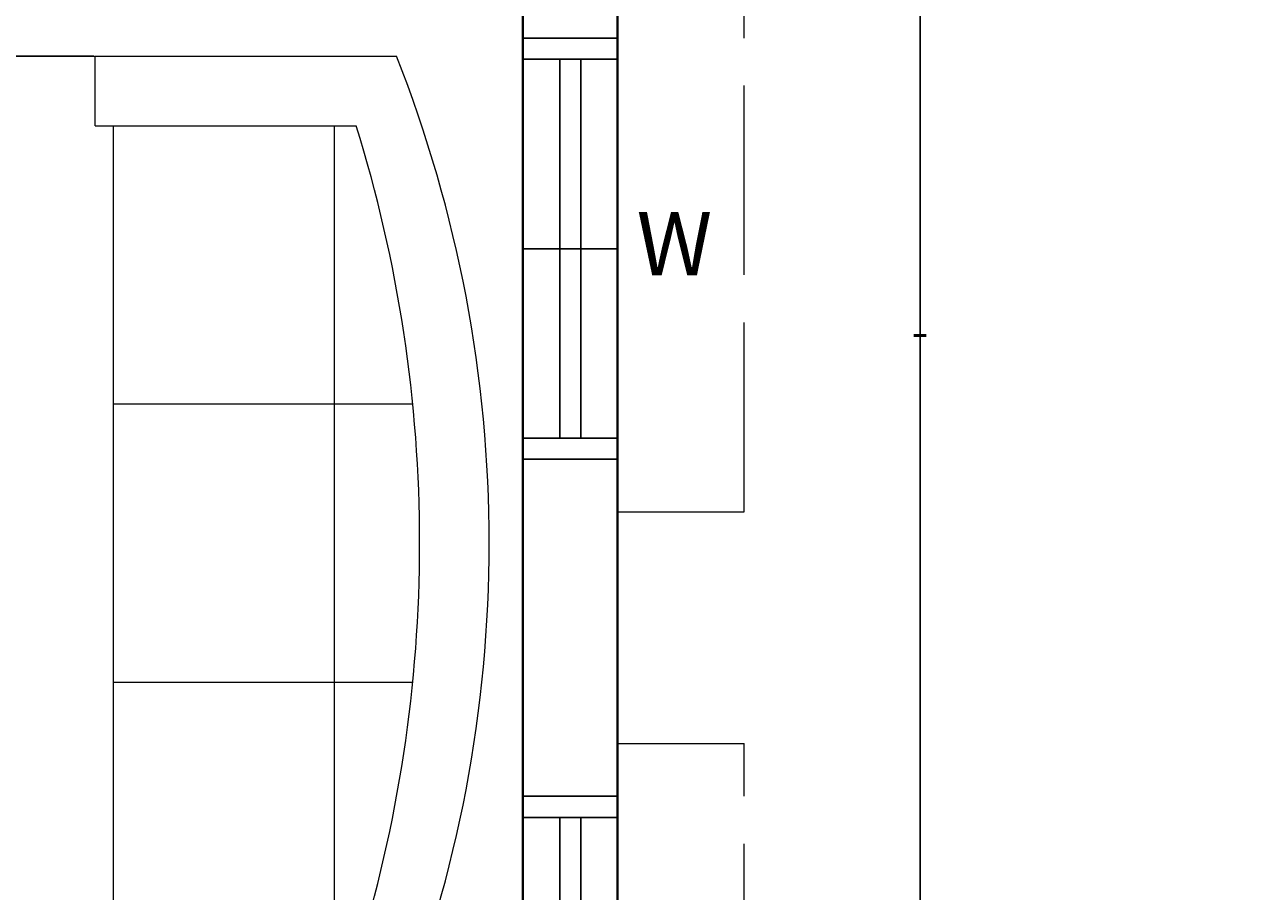
# Model space of a CAD drawing. Units: inches. Extents: x -301 to 715, y -607 to 364.
# Tile 114 of 141: x 77 to 194, y 67 to 149. Entities that reach past the tile are written whole.
import ezdxf

# ---------------------------------------------------------------- set-up
doc = ezdxf.new("R2010")
doc.units = ezdxf.units.IN
doc.header["$MEASUREMENT"] = 0
doc.linetypes.add('ACAD_ISO02W100', pattern=[15, 12, -3])
for name, color, linetype, lineweight in [('A-ANNO-DIMS', 2, 'Continuous', 18), ('A-ANNO-TEXT', 4, 'Continuous', 18), ('A-FURN', 8, 'Continuous', 18), ('A-GLAZ', 2, 'Continuous', 25), ('A-GLAZ-OVHD', 2, 'ACAD_ISO02W100', 18), ('A-WALL', 3, 'Continuous', 40)]:
    doc.layers.add(name, color=color, linetype=linetype, lineweight=lineweight)
doc.styles.get("Standard").update_dxf_attribs({"font": 'arial.ttf'})
doc.dimstyles.get("Standard").update_dxf_attribs({"dimtxt": 0.18, "dimasz": 0.18, "dimexe": 0.18, "dimexo": 0.0625, "dimgap": 0.09, "dimtad": 0, "dimtih": 1, "dimtoh": 1, "dimdec": 1, "dimzin": 0, "dimdsep": 46, "dimlunit": 4, "dimtxsty": 'Standard', "dimcen": 0.09, "dimclrd": 3, "dimclre": 4, "dimclrt": 6, "dimadec": 0, "dimazin": 0, "dimtfac": 1, "dimtdec": 1, "dimtofl": 0, "dimtmove": 0, "dimatfit": 3, "dimfxl": 1, "dimtfill": 2, "dimtfillclr": 51, "dimtolj": 1, "dimtzin": 0, "dimarcsym": 0})

# ---------------------------------------------------------------- blocks, each defined once
blk = doc.blocks.new('Sofa - Roundback 7 ft.')
for p, q in [((-12.00002, -32.4421), (-12.00003, -6.5971)), ((11.99997, -32.4421), (11.99998, -6.5971)), ((-36.000027, -34), (-36.000027, -11.4696)), ((35.99998, -34), (35.99998, -11.4696)), ((-35.999844, -13.3819), (35.9998, -13.3819)), ((-36.000027, -32.4421), (35.99998, -32.4421))]:
    blk.add_line(p, q)
for points in [[(-36.000027, -34), (-42.000027, -34), (-42.000027, -8)], [(41.99998, -8), (41.99998, -34), (35.99998, -34)]]:
    blk.add_lwpolyline(points)
for centre, radius, start, end in [((0, -114.25), 114.25, 68.43141, 111.5686), ((-0.00001, -127.1968), 121.1968, 72.72033, 107.2797)]:
    blk.add_arc(centre, radius, start, end)
blk = doc.blocks.new('WIN-36-PLAN')
for p, q in [((0, 0), (0, 9)), ((2, 0), (2, 9)), ((20, 0), (20, 9)), ((38, 0), (38, 9)), ((40, 0), (40, 9)), ((2, 5.5), (38, 5.5)), ((2, 3.5), (38, 3.5))]:
    blk.add_line(p, q)
blk = doc.blocks.new('WIN-SHADE-50')
at = {"ltscale": 1.5}
for p, q in [((0, 0), (0, 12)), ((50, 12), (0, 12)), ((50, 0), (50, 12)), ((5, 0), (0, 0)), ((45, 0), (50, 0))]:
    blk.add_line(p, q, dxfattribs=at)
blk = doc.blocks.new('*D132')
at = {"layer": 'A-ANNO-DIMS', "color": 4, "lineweight": -2, "transparency": 16777216}
for p, q in [((83.22, 145.95), (69.24, 145.95)), ((83.22, 53.5), (69.24, 53.5))]:
    blk.add_line(p, q, dxfattribs=at)
at = {"layer": 'A-ANNO-DIMS', "color": 3, "lineweight": -2, "transparency": 16777216}
for p, q in [((69.42, 145.77), (69.42, 99.91)), ((69.42, 53.68), (69.42, 99.55))]:
    blk.add_line(p, q, dxfattribs=at)
at = {"layer": 'A-ANNO-DIMS', "color": 3, "transparency": 16777216}
for points in [[(69.39, 145.77), (69.45, 145.77), (69.42, 145.95)], [(69.39, 53.68), (69.45, 53.68), (69.42, 53.5)]]:
    blk.add_solid(points, dxfattribs=at)
at = {"layer": 'Defpoints', "color": 0, "transparency": 16777216}
for p in [(83.29, 145.95), (69.42, 53.5), (83.29, 53.5)]:
    blk.add_point(p, dxfattribs=at)
at = {"layer": 'A-ANNO-DIMS', "color": 6, "transparency": 16777216, "insert": (69.42, 99.73), "char_height": 0.18, "attachment_point": 5, "bg_fill": 1, "box_fill_scale": 1.25, "bg_fill_color": 51, "bg_fill_transparency": 0}
blk.add_mtext('\\A1;SOFA 7\'-8 1/2"', dxfattribs=at)
blk = doc.blocks.new('*D162')
at = {"layer": 'A-ANNO-DIMS', "color": 4, "lineweight": -2, "transparency": 16777216}
for p, q in [((222.33, 320.18), (161.44, 320.18)), ((222.33, -233.82), (161.44, -233.82))]:
    blk.add_line(p, q, dxfattribs=at)
at = {"layer": 'A-ANNO-DIMS', "color": 3, "lineweight": -2, "transparency": 16777216}
for p, q in [((161.62, 320), (161.62, 43.36)), ((161.62, -233.64), (161.62, 43))]:
    blk.add_line(p, q, dxfattribs=at)
at = {"layer": 'A-ANNO-DIMS', "color": 3, "transparency": 16777216}
for points in [[(161.59, 320), (161.65, 320), (161.62, 320.18)], [(161.59, -233.64), (161.65, -233.64), (161.62, -233.82)]]:
    blk.add_solid(points, dxfattribs=at)
at = {"layer": 'Defpoints', "color": 0, "transparency": 16777216}
for p in [(161.62, 320.18), (222.39, 320.18), (222.39, -233.82)]:
    blk.add_point(p, dxfattribs=at)
at = {"layer": 'A-ANNO-DIMS', "color": 6, "transparency": 16777216, "insert": (161.62, 43.18), "char_height": 0.18, "attachment_point": 5, "bg_fill": 1, "box_fill_scale": 1.25, "bg_fill_color": 51, "bg_fill_transparency": 0}
blk.add_mtext('\\A1;46\'-2"', dxfattribs=at)
blk = doc.blocks.new('*D169')
at = {"layer": 'A-ANNO-DIMS', "color": 4, "lineweight": -2, "transparency": 16777216}
for p, q in [((222.33, 183.18), (161.44, 183.18)), ((222.33, 55.68), (161.44, 55.68))]:
    blk.add_line(p, q, dxfattribs=at)
at = {"layer": 'A-ANNO-DIMS', "color": 3, "lineweight": -2, "transparency": 16777216}
for p, q in [((161.62, 183), (161.62, 119.62)), ((161.62, 55.86), (161.62, 119.25))]:
    blk.add_line(p, q, dxfattribs=at)
at = {"layer": 'A-ANNO-DIMS', "color": 3, "transparency": 16777216}
for points in [[(161.59, 183), (161.65, 183), (161.62, 183.18)], [(161.59, 55.86), (161.65, 55.86), (161.62, 55.68)]]:
    blk.add_solid(points, dxfattribs=at)
at = {"layer": 'Defpoints', "color": 0, "transparency": 16777216}
for p in [(161.62, 183.18), (222.39, 183.18), (222.39, 55.68)]:
    blk.add_point(p, dxfattribs=at)
at = {"layer": 'A-ANNO-DIMS', "color": 6, "transparency": 16777216, "insert": (161.62, 119.43), "char_height": 0.18, "attachment_point": 5, "bg_fill": 1, "box_fill_scale": 1.25, "bg_fill_color": 51, "bg_fill_transparency": 0}
blk.add_mtext('\\A1;10\'-7 1/2"', dxfattribs=at)

msp = doc.modelspace()

# ---------------------------------------------------------------- linework, layer by layer
at = {"layer": 'A-WALL'}
for p, q in [((132.9, -9.82), (132.9, 199.18)), ((123.9, -9.82), (123.9, 193.18))]:
    msp.add_line(p, q, dxfattribs=at)

# ---------------------------------------------------------------- block references
at = {"layer": 'A-FURN', "xscale": 1.100593323052692, "yscale": 1.100593323052692, "zscale": 1.100593323052692, "rotation": 270}
msp.add_blockref('Sofa - Roundback 7 ft.', (120.71, 99.73), dxfattribs=at)
at = {"layer": 'A-GLAZ', "rotation": 90.00000000000036}
for p in [(132.9, 107.68), (132.9, 35.68)]:
    msp.add_blockref('WIN-36-PLAN', p, dxfattribs=at)
at = {"layer": 'A-GLAZ-OVHD', "rotation": 270.0000000000001}
for p in [(132.9, 152.68), (132.9, 80.68)]:
    msp.add_blockref('WIN-SHADE-50', p, dxfattribs=at)

# ---------------------------------------------------------------- texts
at = {"layer": 'A-ANNO-TEXT'}
msp.add_text('W', height=6, dxfattribs=at).set_placement((134.7, 125.15))

# ---------------------------------------------------------------- dimensions: what is measured, and where the dimension line sits
at = {"layer": 'A-ANNO-DIMS'}
for base, p1, p2, picture, middle in [((161.62, 320.18), (222.39, -233.82), (222.39, 320.18), '*D162', (161.62, 43.18)), ((161.62, 183.18), (222.39, 55.68), (222.39, 183.18), '*D169', (161.62, 119.43))]:
    dim = msp.add_linear_dim(base=base, p1=p1, p2=p2, angle=90, dimstyle='Standard', override={"dimdec": 1, "dimlfac": 1, "dimrnd": 0, "dimzin": 1, "dimdsep": 46, "dimlunit": 4, "dimfrac": 2}, dxfattribs=at)
    dim.commit()
    dim.dimension.update_dxf_attribs({"geometry": picture, "text_midpoint": middle})
dim = msp.add_linear_dim(base=(69.4192, 53.5044), p1=(83.2867, 145.9543), p2=(83.2867, 53.5044), angle=270, text='SOFA <>', dimstyle='Standard', override={"dimdec": 1, "dimlfac": 1, "dimrnd": 0, "dimzin": 1, "dimdsep": 46, "dimlunit": 4, "dimfrac": 2}, dxfattribs=at)
dim.commit()
dim.dimension.update_dxf_attribs({"geometry": '*D132', "text_midpoint": (69.4192, 99.7293)})

doc.saveas('drawing.dxf')
